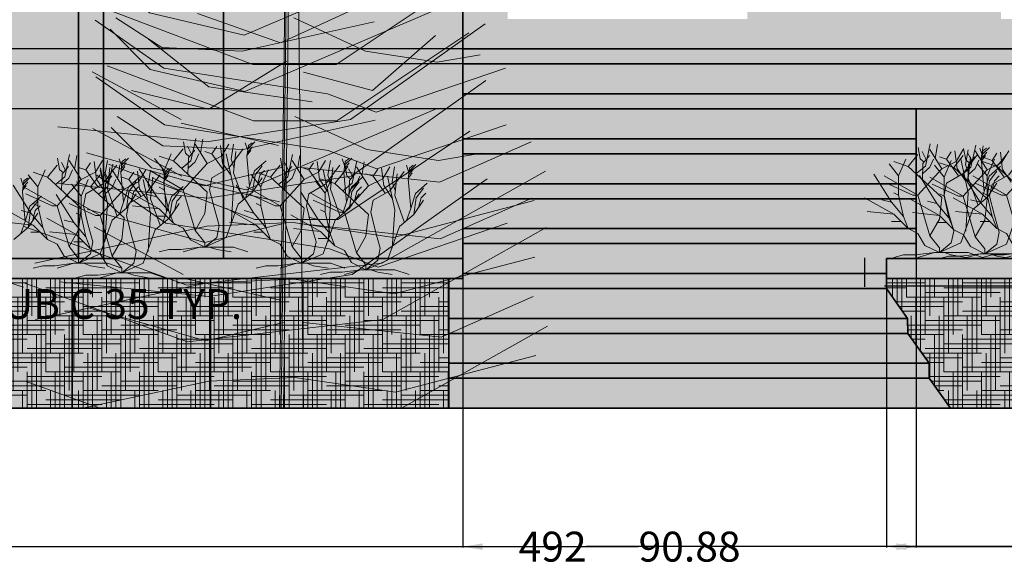
# Model space of a CAD drawing. Units: inches. Extents: x 221 to 874, y 171 to 738.
# Tile 5 of 11: x 452 to 650, y 171 to 281. Entities that reach past the tile are written whole.
import ezdxf

# ---------------------------------------------------------------- set-up
doc = ezdxf.new("R2010")
doc.units = ezdxf.units.IN
doc.header["$MEASUREMENT"] = 0
for name, color, linetype, lineweight in [('A-ANNO-DIMS', 2, 'Continuous', 18), ('A-ELEV', 7, 'Continuous', 35), ('A-ELEV-PATT', 8, 'Continuous', 13), ('L-PLNT', 3, 'Continuous', 13)]:
    doc.layers.add(name, color=color, linetype=linetype, lineweight=lineweight)
doc.styles.get("Standard").update_dxf_attribs({"font": 'arial.ttf'})
doc.dimstyles.get("Standard").update_dxf_attribs({"dimtxt": 6, "dimasz": 4, "dimexe": 0.18, "dimexo": 0.0625, "dimgap": 0.09, "dimtad": 0, "dimtih": 1, "dimtoh": 1, "dimdec": 0, "dimzin": 0, "dimdsep": 46, "dimlunit": 3, "dimtxsty": 'Standard', "dimcen": 0.09, "dimadec": 0, "dimazin": 0, "dimtfac": 1, "dimtdec": 0, "dimtofl": 0, "dimtmove": 0, "dimatfit": 3, "dimfxl": 1, "dimtolj": 1, "dimtzin": 0, "dimarcsym": 0})

# ---------------------------------------------------------------- blocks, each defined once
blk = doc.blocks.new('SHRUB-A')
for p, q in [((8.78, 18.24), (10.7, 20.64)), ((15.5, 17.76), (13.1, 21.6)), ((18.38, 19.2), (19.82, 21.6)), ((19.82, 16.8), (22.7, 20.64)), ((6.86, 16.32), (4.94, 18.72)), ((8.78, 18.24), (5.9, 19.2)), ((6.86, 16.32), (8.3, 19.68)), ((15.5, 12), (8.78, 18.24)), ((10.7, 12.48), (15.5, 17.76)), ((15.5, 17.76), (18.38, 19.2)), ((5.42, 11.04), (1.91, 16.66)), ((10.7, 12.48), (3.98, 16.32)), ((6.86, 12.48), (6.86, 16.32)), ((16.46, 14.88), (19.82, 16.8)), ((25.1, 15.36), (26.54, 17.28)), ((9.74, 12.48), (4.46, 14.88)), ((15.98, 12.48), (16.46, 14.88)), ((24.62, 12), (25.1, 15.36)), ((24.62, 12), (26.54, 14.88)), ((5.9, 8.64), (0, 11.96)), ((6.86, 12.48), (5.9, 12.96)), ((7.82, 8.16), (6.86, 12.48)), ((10.7, 12.48), (9.74, 12.48)), ((13.1, 4.32), (10.7, 12.48)), ((15.02, 7.68), (15.5, 12)), ((16.94, 8.64), (15.98, 12.48)), ((21.74, 9.6), (24.62, 12)), ((5.42, 11.04), (3.5, 11.52)), ((7.82, 8.16), (5.42, 11.04)), ((5.9, 8.64), (0.53, 9.22)), ((8.78, 5.76), (5.9, 8.64)), ((8.78, 5.76), (7.82, 8.16)), ((17.9, 5.28), (16.94, 8.64)), ((19.34, 2.88), (21.74, 9.6)), ((13.1, 4.32), (15.02, 7.68)), ((10.7, 4.8), (8.78, 5.76)), ((12.14, 2.4), (10.7, 4.8)), ((15.02, 1.92), (13.1, 4.32)), ((17.42, 2.88), (17.9, 5.28)), ((15.02, 0.96), (12.14, 2.4)), ((15.02, 0.96), (19.34, 2.88)), ((15.02, 0.96), (17.42, 2.88)), ((15.02, 0.96), (15.02, 1.92)), ((15.02, 0.96), (20.78, 0.96)), ((20.78, 0.96), (23.66, 0))]:
    blk.add_line(p, q)
blk = doc.blocks.new('GRASS-TUFT')
for p, q in [((0.28, 8.35), (0.58, 10.54)), ((0.58, 10.54), (1.31, 11.09)), ((0.83, 2.4), (0.28, 8.35)), ((1.8, 5.45), (4.12, 7.49)), ((0.83, 2.4), (1.8, 5.45)), ((0, 0), (0.83, 2.4))]:
    blk.add_line(p, q)
blk = doc.blocks.new('SHRUB-B')
for p, q in [((8.78, 18.24), (10.7, 20.64)), ((15.5, 17.76), (13.1, 21.6)), ((18.38, 19.2), (19.82, 21.6)), ((19.82, 16.8), (22.7, 20.64)), ((6.86, 16.32), (4.94, 18.72)), ((8.78, 18.24), (5.9, 19.2)), ((6.86, 16.32), (8.3, 19.68)), ((15.5, 12), (8.78, 18.24)), ((10.7, 12.48), (15.5, 17.76)), ((15.5, 17.76), (18.38, 19.2)), ((5.42, 11.04), (1.91, 16.66)), ((10.7, 12.48), (3.98, 16.32)), ((6.86, 12.48), (6.86, 16.32)), ((16.46, 14.88), (19.82, 16.8)), ((25.1, 15.36), (26.54, 17.28)), ((9.74, 12.48), (4.46, 14.88)), ((15.98, 12.48), (16.46, 14.88)), ((24.62, 12), (25.1, 15.36)), ((24.62, 12), (26.54, 14.88)), ((5.9, 8.64), (0, 11.96)), ((6.86, 12.48), (5.9, 12.96)), ((7.82, 8.16), (6.86, 12.48)), ((10.7, 12.48), (9.74, 12.48)), ((13.1, 4.32), (10.7, 12.48)), ((15.02, 7.68), (15.5, 12)), ((16.94, 8.64), (15.98, 12.48)), ((21.74, 9.6), (24.62, 12)), ((5.42, 11.04), (3.5, 11.52)), ((7.82, 8.16), (5.42, 11.04)), ((5.9, 8.64), (0.53, 9.22)), ((8.78, 5.76), (5.9, 8.64)), ((8.78, 5.76), (7.82, 8.16)), ((17.9, 5.28), (16.94, 8.64)), ((19.34, 2.88), (21.74, 9.6)), ((13.1, 4.32), (15.02, 7.68)), ((10.7, 4.8), (8.78, 5.76)), ((12.14, 2.4), (10.7, 4.8)), ((15.02, 1.92), (13.1, 4.32)), ((17.42, 2.88), (17.9, 5.28)), ((15.02, 0.96), (12.14, 2.4)), ((15.02, 0.96), (19.34, 2.88)), ((15.02, 0.96), (17.42, 2.88)), ((15.02, 0.96), (15.02, 1.92)), ((15.02, 0.96), (20.78, 0.96)), ((20.78, 0.96), (23.66, 0)), ((25.58, 0.48), (23.66, 0)), ((27.98, 0.48), (25.58, 0.48)), ((31.82, 0.96), (27.98, 0.48)), ((31.82, 0.96), (28.46, 0)), ((31.82, 0.96), (33.74, 0.96)), ((33.74, 0.96), (35.18, 0.48)), ((35.18, 0.48), (38.06, 0))]:
    blk.add_line(p, q)
blk = doc.blocks.new('GRASS-SPRIG')
for p, q in [((1.44, 3.36), (2.4, 4.8)), ((1.44, 3.36), (0, 3.84)), ((3.84, 0), (1.44, 3.36))]:
    blk.add_line(p, q)
blk = doc.blocks.new('SHRUB-C')
for p, q in [((8.78, 20.16), (10.7, 22.56)), ((15.5, 19.68), (13.1, 23.52)), ((18.38, 21.12), (19.82, 23.52)), ((19.82, 18.72), (22.7, 22.56)), ((6.86, 18.24), (4.94, 20.64)), ((8.78, 20.16), (5.9, 21.12)), ((6.86, 18.24), (8.3, 21.6)), ((15.5, 13.92), (8.78, 20.16)), ((15.5, 19.68), (18.38, 21.12)), ((17.42, 18.24), (19.34, 20.64)), ((24.14, 17.76), (21.74, 21.6)), ((27.02, 19.2), (28.46, 21.6)), ((28.46, 16.8), (31.34, 20.64)), ((5.42, 12.96), (1.91, 18.58)), ((10.7, 14.4), (3.98, 18.24)), ((6.86, 14.4), (6.86, 18.24)), ((10.7, 14.4), (15.5, 19.68)), ((15.5, 16.32), (13.58, 18.72)), ((17.42, 18.24), (14.54, 19.2)), ((15.5, 16.32), (16.94, 19.68)), ((16.46, 16.8), (19.82, 18.72)), ((24.14, 12), (17.42, 18.24)), ((19.34, 12.48), (24.14, 17.76)), ((24.14, 17.76), (27.02, 19.2)), ((25.1, 17.28), (26.54, 19.2)), ((9.74, 14.4), (4.46, 16.8)), ((14.06, 11.04), (10.55, 16.66)), ((19.34, 12.48), (12.62, 16.32)), ((15.5, 12.48), (15.5, 16.32)), ((15.98, 14.4), (16.46, 16.8)), ((24.62, 13.92), (25.1, 17.28)), ((24.62, 13.92), (26.54, 16.8)), ((25.1, 14.88), (28.46, 16.8)), ((33.74, 15.36), (35.18, 17.28)), ((5.9, 10.56), (0, 13.88)), ((6.86, 14.4), (5.9, 14.88)), ((7.82, 10.08), (6.86, 14.4)), ((10.7, 14.4), (9.74, 14.4)), ((13.1, 6.24), (10.7, 14.4)), ((18.38, 12.48), (13.1, 14.88)), ((15.02, 9.6), (15.5, 13.92)), ((16.94, 10.56), (15.98, 14.4)), ((21.74, 11.52), (24.62, 13.92)), ((24.62, 12.48), (25.1, 14.88)), ((33.26, 12), (33.74, 15.36)), ((33.26, 12), (35.18, 14.88)), ((5.42, 12.96), (3.5, 13.44)), ((7.82, 10.08), (5.42, 12.96)), ((14.54, 8.64), (8.64, 11.96)), ((15.5, 12.48), (14.54, 12.96)), ((16.46, 8.16), (15.5, 12.48)), ((19.34, 12.48), (18.38, 12.48)), ((21.74, 4.32), (19.34, 12.48)), ((23.66, 7.68), (24.14, 12)), ((25.58, 8.64), (24.62, 12.48)), ((30.38, 9.6), (33.26, 12)), ((5.9, 10.56), (0.53, 11.14)), ((8.78, 7.68), (5.9, 10.56)), ((8.78, 7.68), (7.82, 10.08)), ((14.06, 11.04), (12.14, 11.52)), ((16.46, 8.16), (14.06, 11.04)), ((17.9, 7.2), (16.94, 10.56)), ((19.34, 4.8), (21.74, 11.52)), ((14.54, 8.64), (9.17, 9.22)), ((13.1, 6.24), (15.02, 9.6)), ((17.42, 5.76), (14.54, 8.64)), ((17.42, 5.76), (16.46, 8.16)), ((26.54, 5.28), (25.58, 8.64)), ((27.98, 2.88), (30.38, 9.6)), ((10.7, 6.72), (8.78, 7.68)), ((12.14, 4.32), (10.7, 6.72)), ((15.02, 3.84), (13.1, 6.24)), ((17.42, 4.8), (17.9, 7.2)), ((21.74, 4.32), (23.66, 7.68)), ((15.02, 2.88), (12.14, 4.32)), ((15.02, 2.88), (19.34, 4.8)), ((15.02, 2.88), (17.42, 4.8)), ((19.34, 4.8), (17.42, 5.76)), ((20.78, 2.4), (19.34, 4.8)), ((23.66, 1.92), (21.74, 4.32)), ((26.06, 2.88), (26.54, 5.28)), ((15.02, 2.88), (15.02, 3.84)), ((15.02, 2.88), (20.78, 2.88)), ((20.78, 2.88), (23.66, 1.92)), ((23.66, 0.96), (20.78, 2.4)), ((23.66, 0.96), (27.98, 2.88)), ((23.66, 0.96), (26.06, 2.88)), ((23.66, 0.96), (23.66, 1.92)), ((23.66, 0.96), (29.42, 0.96)), ((29.42, 0.96), (32.3, 0))]:
    blk.add_line(p, q)
blk = doc.blocks.new('*D16')
at = {"layer": 'A-ANNO-DIMS', "color": 0, "lineweight": -2, "transparency": 16777216}
for p, q in [((621.56, 232.89), (621.56, 227.07)), ((659.62, 232.89), (659.62, 227.07)), ((625.56, 227.25), (655.62, 227.25)), ((659.62, 227.25), (663.62, 227.25))]:
    blk.add_line(p, q, dxfattribs=at)
at = {"layer": 'A-ANNO-DIMS', "color": 0, "transparency": 16777216}
for points in [[(625.56, 227.91), (625.56, 226.58), (621.56, 227.25)], [(655.62, 227.91), (655.62, 226.58), (659.62, 227.25)]]:
    blk.add_solid(points, dxfattribs=at)
at = {"layer": 'Defpoints', "color": 0, "transparency": 16777216}
for p in [(621.56, 232.96), (659.62, 232.96), (659.62, 227.25)]:
    blk.add_point(p, dxfattribs=at)
at = {"layer": 'A-ANNO-DIMS', "color": 0, "transparency": 16777216, "insert": (698.1, 227.25), "char_height": 6, "attachment_point": 5}
blk.add_mtext('\\A1;SHRUB B 38 TYP.', dxfattribs=at)
blk = doc.blocks.new('*D18')
at = {"layer": 'A-ANNO-DIMS', "color": 0, "lineweight": -2, "transparency": 16777216}
for p, q in [((391.06, 228.81), (391.06, 223.42)), ((426.24, 228.81), (426.24, 223.42)), ((395.06, 223.6), (422.24, 223.6)), ((426.24, 223.6), (430.24, 223.6))]:
    blk.add_line(p, q, dxfattribs=at)
at = {"layer": 'A-ANNO-DIMS', "color": 0, "transparency": 16777216}
for points in [[(395.06, 224.27), (395.06, 222.93), (391.06, 223.6)], [(422.24, 224.27), (422.24, 222.93), (426.24, 223.6)]]:
    blk.add_solid(points, dxfattribs=at)
at = {"layer": 'Defpoints', "color": 0, "transparency": 16777216}
for p in [(391.06, 228.88), (426.24, 228.88), (426.24, 223.6)]:
    blk.add_point(p, dxfattribs=at)
at = {"layer": 'A-ANNO-DIMS', "color": 0, "transparency": 16777216, "insert": (464.94, 223.6), "char_height": 6, "attachment_point": 5}
blk.add_mtext('\\A1;SHRUB C 35 TYP.', dxfattribs=at)
blk = doc.blocks.new('*D20')
at = {"layer": 'A-ANNO-DIMS', "color": 0, "lineweight": -2, "transparency": 16777216}
for p, q in [((313.08, 202.65), (313.08, 174.79)), ((805.08, 202.65), (805.08, 174.79)), ((317.08, 174.97), (552.27, 174.97)), ((801.08, 174.97), (565.89, 174.97))]:
    blk.add_line(p, q, dxfattribs=at)
at = {"layer": 'A-ANNO-DIMS', "color": 0, "transparency": 16777216}
for points in [[(317.08, 175.63), (317.08, 174.3), (313.08, 174.97)], [(801.08, 175.63), (801.08, 174.3), (805.08, 174.97)]]:
    blk.add_solid(points, dxfattribs=at)
at = {"layer": 'Defpoints', "color": 0, "transparency": 16777216}
for p in [(313.08, 202.72), (805.08, 202.72), (805.08, 174.97)]:
    blk.add_point(p, dxfattribs=at)
at = {"layer": 'A-ANNO-DIMS', "color": 0, "transparency": 16777216, "insert": (559.08, 174.97), "char_height": 6, "attachment_point": 5}
blk.add_mtext('\\A1;492', dxfattribs=at)
blk = doc.blocks.new('*D21')
at = {"layer": 'A-ANNO-DIMS', "color": 0, "lineweight": -2, "transparency": 16777216}
for p, q in [((541.14, 706.72), (833.01, 706.72)), ((832.83, 702.72), (832.83, 457.87)), ((832.83, 206.72), (832.83, 451.56)), ((805.14, 202.72), (833.01, 202.72))]:
    blk.add_line(p, q, dxfattribs=at)
at = {"layer": 'A-ANNO-DIMS', "color": 0, "transparency": 16777216}
for points in [[(832.16, 702.72), (833.5, 702.72), (832.83, 706.72)], [(832.16, 206.72), (833.5, 206.72), (832.83, 202.72)]]:
    blk.add_solid(points, dxfattribs=at)
at = {"layer": 'Defpoints', "color": 0, "transparency": 16777216}
for p in [(541.08, 706.72), (832.83, 706.72), (805.08, 202.72)]:
    blk.add_point(p, dxfattribs=at)
at = {"layer": 'A-ANNO-DIMS', "color": 0, "transparency": 16777216, "insert": (832.83, 454.72), "char_height": 6, "attachment_point": 5}
blk.add_mtext('\\A1;504', dxfattribs=at)
blk = doc.blocks.new('*D67')
at = {"layer": 'A-ANNO-DIMS', "color": 0, "lineweight": -2, "transparency": 16777216}
for p, q in [((231.54, 271.72), (231.54, 275.72)), ((231.54, 275.72), (235.54, 275.72)), ((541.02, 271.72), (231.36, 271.72)), ((231.54, 266.72), (231.54, 267.72)), ((541.02, 262.72), (231.36, 262.72))]:
    blk.add_line(p, q, dxfattribs=at)
at = {"layer": 'A-ANNO-DIMS', "color": 0, "transparency": 16777216}
for points in [[(230.88, 267.72), (232.21, 267.72), (231.54, 271.72)], [(230.88, 266.72), (232.21, 266.72), (231.54, 262.72)]]:
    blk.add_solid(points, dxfattribs=at)
at = {"layer": 'Defpoints', "color": 0, "transparency": 16777216}
for p in [(231.54, 271.72), (541.08, 271.72), (541.08, 262.72)]:
    blk.add_point(p, dxfattribs=at)
at = {"layer": 'A-ANNO-DIMS', "color": 0, "transparency": 16777216, "insert": (237.61, 275.72), "char_height": 6, "attachment_point": 5}
blk.add_mtext('\\A1;9', dxfattribs=at)
blk = doc.blocks.new('*D68')
at = {"layer": 'A-ANNO-DIMS', "color": 0, "lineweight": -2, "transparency": 16777216}
for p, q in [((231.54, 278.72), (231.54, 282.72)), ((231.54, 282.72), (235.54, 282.72)), ((541.02, 274.72), (231.36, 274.72)), ((541.02, 271.72), (231.36, 271.72)), ((231.54, 267.72), (231.54, 263.72))]:
    blk.add_line(p, q, dxfattribs=at)
at = {"layer": 'A-ANNO-DIMS', "color": 0, "transparency": 16777216}
for points in [[(230.88, 278.72), (232.21, 278.72), (231.54, 274.72)], [(230.88, 267.72), (232.21, 267.72), (231.54, 271.72)]]:
    blk.add_solid(points, dxfattribs=at)
at = {"layer": 'Defpoints', "color": 0, "transparency": 16777216}
for p in [(231.54, 274.72), (541.08, 274.72), (541.08, 271.72)]:
    blk.add_point(p, dxfattribs=at)
at = {"layer": 'A-ANNO-DIMS', "color": 0, "transparency": 16777216, "insert": (237.6, 282.72), "char_height": 6, "attachment_point": 5}
blk.add_mtext('\\A1;3', dxfattribs=at)
blk = doc.blocks.new('*D69')
at = {"layer": 'A-ANNO-DIMS', "color": 0, "lineweight": -2, "transparency": 16777216}
for p, q in [((541.08, 262.65), (541.08, 174.79)), ((631.96, 262.65), (631.96, 174.79)), ((545.08, 174.97), (576.3, 174.97)), ((627.96, 174.97), (596.74, 174.97))]:
    blk.add_line(p, q, dxfattribs=at)
at = {"layer": 'A-ANNO-DIMS', "color": 0, "transparency": 16777216}
for points in [[(545.08, 175.63), (545.08, 174.3), (541.08, 174.97)], [(627.96, 175.63), (627.96, 174.3), (631.96, 174.97)]]:
    blk.add_solid(points, dxfattribs=at)
at = {"layer": 'Defpoints', "color": 0, "transparency": 16777216}
for p in [(541.08, 262.72), (631.96, 262.72), (631.96, 174.97)]:
    blk.add_point(p, dxfattribs=at)
at = {"layer": 'A-ANNO-DIMS', "color": 0, "transparency": 16777216, "insert": (586.52, 174.97), "char_height": 6, "attachment_point": 5}
blk.add_mtext('\\A1;90.88', dxfattribs=at)
blk = doc.blocks.new('*D70')
at = {"layer": 'A-ANNO-DIMS', "color": 0, "lineweight": -2, "transparency": 16777216}
for p, q in [((625.96, 229.65), (625.96, 174.79)), ((805.08, 202.65), (805.08, 174.79)), ((629.96, 174.97), (703.29, 174.97)), ((801.08, 174.97), (727.75, 174.97))]:
    blk.add_line(p, q, dxfattribs=at)
at = {"layer": 'A-ANNO-DIMS', "color": 0, "transparency": 16777216}
for points in [[(629.96, 175.63), (629.96, 174.3), (625.96, 174.97)], [(801.08, 175.63), (801.08, 174.3), (805.08, 174.97)]]:
    blk.add_solid(points, dxfattribs=at)
at = {"layer": 'Defpoints', "color": 0, "transparency": 16777216}
for p in [(625.96, 229.72), (805.08, 202.72), (805.08, 174.97)]:
    blk.add_point(p, dxfattribs=at)
at = {"layer": 'A-ANNO-DIMS', "color": 0, "transparency": 16777216, "insert": (715.52, 174.97), "char_height": 6, "attachment_point": 5}
blk.add_mtext('\\A1;179.12', dxfattribs=at)

msp = doc.modelspace()

# ---------------------------------------------------------------- hatches: boundary and pattern name
at = {"layer": 'A-ELEV-PATT'}
h = msp.add_hatch(color=256, dxfattribs=at)
h.dxf.hatch_style = 1
h.paths.add_polyline_path([(349.0786, 286.1996), (313.0786, 286.1996), (313.0786, 232.7164), (349.0786, 232.7164)])
h.paths.add_polyline_path([(464.0786, 286.1996), (406.0786, 286.1996), (406.0786, 232.7164), (464.0786, 232.7164)])
h.paths.add_polyline_path([(541.0786, 286.1996), (493.0786, 286.1996), (493.0786, 232.7164), (541.0786, 232.7164)])
h.paths.add_polyline_path([(541.0786, 370.7164), (493.0786, 370.7164), (493.0786, 286.1996), (541.0786, 286.1996)])
h.paths.add_polyline_path([(464.0786, 370.7164), (406.0786, 370.7164), (406.0786, 286.1996), (464.0786, 286.1996)])
h.paths.add_polyline_path([(349.0786, 370.7164), (313.0786, 370.7164), (313.0786, 286.1996), (349.0786, 286.1996)])
h.paths.add_polyline_path([(349.0786, 454.7164), (313.0786, 454.7164), (313.0786, 370.7164), (349.0786, 370.7164)])
h.paths.add_polyline_path([(464.0786, 454.7164), (406.0786, 454.7164), (406.0786, 370.7164), (464.0786, 370.7164)])
h.paths.add_polyline_path([(541.0786, 418.7164), (541.0786, 454.7164), (493.0786, 454.7164), (493.0786, 370.7164), (541.0786, 370.7164)])
h.paths.add_polyline_path([(541.0786, 550.7164), (493.0786, 550.7164), (493.0786, 454.7164), (541.0786, 454.7164)])
h.paths.add_polyline_path([(464.0786, 550.7164), (406.0786, 550.7164), (406.0786, 454.7164), (464.0786, 454.7164)])
h.paths.add_polyline_path([(349.0786, 550.7164), (313.0786, 550.7164), (313.0786, 454.7164), (349.0786, 454.7164)])
h.paths.add_polyline_path([(349.0786, 586.7164), (313.0786, 586.7164), (313.0786, 550.7164), (349.0786, 550.7164)])
h.paths.add_polyline_path([(464.0786, 586.7164), (406.0786, 586.7164), (406.0786, 550.7164), (464.0786, 550.7164)])
h.paths.add_polyline_path([(541.0786, 574.7164), (541.0786, 586.7164), (493.0786, 586.7164), (493.0786, 550.7164), (541.0786, 550.7164)])
h.paths.add_polyline_path([(541.0786, 670.7164), (493.0786, 670.7164), (493.0786, 586.7164), (541.0786, 586.7164)])
h.paths.add_polyline_path([(464.0786, 670.7164), (406.0786, 670.7164), (406.0786, 586.7164), (464.0786, 586.7164)])
h.paths.add_polyline_path([(349.0786, 670.7164), (313.0786, 670.7164), (313.0786, 586.7164), (349.0786, 586.7164)])
h.paths.add_polyline_path([(406.0786, 706.7164), (313.0786, 706.7164), (313.0786, 670.7164), (349.0786, 670.7164), (406.0786, 670.7164)])
h.paths.add_polyline_path([(464.0786, 706.7164), (406.0786, 706.7164), (406.0786, 670.7164), (464.0786, 670.7164)])
h.paths.add_polyline_path([(541.0786, 706.7164), (493.0786, 706.7164), (493.0786, 688.7164), (493.0786, 670.7164), (541.0786, 670.7164)])
h.paths.add_polyline_path([(660.0786, 610.7164), (541.0786, 610.7164), (541.0786, 586.7164), (541.0786, 574.7164), (660.0786, 574.7164)])
h.paths.add_polyline_path([(781.0786, 610.7164), (660.0786, 610.7164), (660.0786, 574.7164), (769.0786, 574.7164), (781.0786, 574.7164)])
h.paths.add_polyline_path([(781.0786, 574.7164), (769.0786, 574.7164), (769.0786, 476.1199), (781.0786, 476.1199)])
h.paths.add_polyline_path([(781.0786, 476.1199), (769.0786, 476.1199), (769.0786, 457.7164), (781.0786, 457.7164)])
h.paths.add_polyline_path([(781.0786, 377.1023), (705.9097, 377.1023), (705.9097, 286.1996), (781.0786, 286.1996)])
h.paths.add_polyline_path([(741.9618, 338.8486), (756.9618, 338.8486), (756.9618, 329.8486), (741.9618, 329.8486)], flags=16)
h.paths.add_polyline_path([(648.9097, 377.1023), (598.0786, 377.1023), (598.0786, 286.1996), (648.9097, 286.1996)])
h.paths.add_polyline_path([(781.0786, 286.1996), (705.9097, 286.1996), (705.9097, 280.7164), (648.9097, 280.7164), (648.9097, 286.1996), (598.0786, 286.1996), (598.0786, 280.7164), (550.0786, 280.7164), (550.0786, 286.1996), (541.0786, 286.1996), (541.0786, 274.7164), (781.0786, 274.7164)])
h.paths.add_polyline_path([(660.0786, 562.7164), (546.3477, 562.7164), (546.3477, 457.7164), (660.0786, 457.7164)])
h = msp.add_hatch(color=256, dxfattribs=at)
h.set_gradient(color1=(255, 236, 199), name='CYLINDER')
h.paths.add_polyline_path([(469.0786, 680.7164), (464.0786, 680.7164), (464.0786, 232.7164), (469.0786, 232.7164)])
h = msp.add_hatch(color=256, dxfattribs=at)
h.set_gradient(color1=(99, 100, 102), color2=(254, 234, 185), name='INVCYLINDER')
h.paths.add_polyline_path([(493.0786, 426.7164), (469.0786, 426.7164), (469.0786, 232.7164), (493.0786, 232.7164)])
h = msp.add_hatch(color=256, dxfattribs=at)
h.set_gradient(color1=(99, 100, 102), color2=(169, 160, 132), name='INVCYLINDER')
h.paths.add_polyline_path([(541.0786, 274.7164), (541.0786, 271.7164), (787.0786, 271.7164), (781.0786, 274.7164)])
h = msp.add_hatch(color=256, dxfattribs=at)
h.paths.add_polyline_path([(787.0786, 271.7164), (541.0786, 271.7164), (541.0786, 265.7164), (799.0786, 265.7164)])
h.paths.add_polyline_path([(631.9596, 262.7164), (541.0786, 262.7164), (541.0786, 256.7164), (631.9596, 256.7164)])
h.paths.add_polyline_path([(631.9596, 253.7164), (541.0786, 253.7164), (541.0786, 247.7164), (631.9596, 247.7164)])
h.paths.add_polyline_path([(631.9596, 244.7164), (541.0786, 244.7164), (541.0786, 238.7164), (631.9596, 238.7164)])
h.paths.add_polyline_path([(631.9596, 235.7164), (541.0786, 235.7164), (541.0786, 229.7164), (625.9596, 229.7164), (625.9596, 232.7164), (631.9596, 232.7164)])
h.paths.add_polyline_path([(630.2472, 217.7164), (538.2859, 217.7164), (538.2859, 211.7164), (634.5124, 211.7164), (634.5123, 211.7326)], flags=17)
h.paths.add_polyline_path([(634.5396, 208.7164), (538.2859, 208.7164), (538.2859, 202.7164), (638.8162, 202.7164)])
h = msp.add_hatch(color=256, dxfattribs=at)
h.set_gradient(color1=(99, 100, 102), color2=(248, 246, 176), name='CYLINDER')
h.paths.add_polyline_path([(805.0786, 262.7164), (799.0786, 265.7164), (541.0786, 265.7164), (541.0786, 262.7164)])
for points in [[(631.9596, 262.7164), (631.9596, 232.7164), (805.0786, 232.7164), (805.0786, 262.7164)], [(313.0786, 232.7164), (313.0786, 228.7164), (541.0786, 228.7164), (541.0786, 232.7164)], [(805.0786, 228.7164), (805.0786, 232.7164), (625.9596, 232.7164), (625.9596, 228.7164)], [(538.2859, 226.7164), (538.2859, 220.7164), (630.2279, 220.7164), (625.9626, 226.7164)]]:
    msp.add_hatch(color=256, dxfattribs=at).paths.add_polyline_path(points)
h = msp.add_hatch(color=256, dxfattribs=at)
h.set_gradient(color1=(99, 100, 102), color2=(248, 246, 176), name='CYLINDER')
h.paths.add_polyline_path([(541.0786, 256.7164), (541.0786, 253.7164), (631.9596, 253.7164), (631.9596, 256.7164)])
h = msp.add_hatch(color=256, dxfattribs=at)
h.set_gradient(color1=(99, 100, 102), color2=(248, 246, 176), name='CYLINDER')
h.paths.add_polyline_path([(541.0786, 247.7164), (541.0786, 244.7164), (631.9596, 244.7164), (631.9596, 247.7164)])
h = msp.add_hatch(color=256, dxfattribs=at)
h.set_gradient(color1=(99, 100, 102), color2=(248, 246, 176), name='CYLINDER')
h.paths.add_polyline_path([(631.9596, 235.7164), (631.9596, 238.7164), (541.0786, 238.7164), (541.0786, 235.7164)])
h = msp.add_hatch(color=256, dxfattribs=at)
h.set_gradient(color1=(99, 100, 102), color2=(248, 246, 176), name='CYLINDER')
h.paths.add_polyline_path([(625.9626, 226.7164), (625.9606, 228.7164), (625.9596, 228.7164), (625.9596, 229.7164), (541.0786, 229.7164), (541.0786, 228.7164), (538.2859, 228.7164), (538.2859, 226.7164)])
h = msp.add_hatch(color=256, dxfattribs=at)
h.set_gradient(color1=(147, 149, 152), color2=(91, 91, 91), name='CURVED')
h.paths.add_polyline_path([(462.8078, 202.7164), (462.8078, 228.7164), (414.8291, 228.7164), (414.8291, 202.7164)])
h = msp.add_hatch(dxfattribs=at)
h.set_pattern_fill('HOUND', color=256, scale=15, style=0)
h.paths.add_polyline_path([(462.8078, 228.7164), (414.8291, 228.7164), (414.8291, 202.7164), (462.8078, 202.7164)])
h = msp.add_hatch(color=256, dxfattribs=at)
h.set_gradient(color1=(99, 100, 102), color2=(91, 91, 91), rotation=180, name='INVCURVED')
h.paths.add_polyline_path([(462.8078, 202.7164), (490.5003, 202.7164), (490.5003, 228.7164), (462.8078, 228.7164)])
h = msp.add_hatch(dxfattribs=at)
h.set_pattern_fill('HOUND', color=256, scale=15, style=0)
h.paths.add_polyline_path([(490.5003, 228.7164), (462.8078, 228.7164), (462.8078, 202.7164), (490.5003, 202.7164)])
h = msp.add_hatch(color=256, dxfattribs=at)
h.set_gradient(color1=(147, 149, 152), color2=(91, 91, 91), name='CURVED')
h.paths.add_polyline_path([(538.2859, 202.7164), (538.2859, 228.7164), (490.5003, 228.7164), (490.5003, 202.7164)])
h = msp.add_hatch(dxfattribs=at)
h.set_pattern_fill('HOUND', color=256, scale=15, style=0)
h.paths.add_polyline_path([(538.2859, 228.7164), (490.5003, 228.7164), (490.5003, 202.7164), (538.2859, 202.7164)])
h = msp.add_hatch(color=256, dxfattribs=at)
h.set_gradient(color1=(147, 149, 152), color2=(99, 100, 102), name='CURVED')
h.paths.add_polyline_path([(656.1863, 228.7164), (625.9606, 228.7164), (625.9626, 226.7164), (630.2279, 220.7164), (630.2471, 217.7164), (634.5238, 211.7164), (634.5124, 211.7164), (634.5315, 208.7276), (638.8162, 202.7164), (656.1863, 202.7164)])
h = msp.add_hatch(dxfattribs=at)
h.set_pattern_fill('HOUND', color=256, scale=15, style=0)
h.paths.add_polyline_path([(656.1863, 228.7164), (625.9606, 228.7164), (625.9626, 226.7164), (630.2279, 220.7164), (630.2471, 217.7164), (634.5238, 211.7164), (634.5124, 211.7164), (634.5315, 208.7276), (638.8162, 202.7164), (656.1863, 202.7164)])
h = msp.add_hatch(color=256, dxfattribs=at)
h.set_gradient(color1=(99, 100, 102), color2=(248, 246, 176), name='CYLINDER')
h.paths.add_polyline_path([(630.2471, 217.7164), (630.2279, 220.7164), (538.2859, 220.7164), (538.2859, 217.7164)])
h.paths.add_polyline_path([(634.5316, 208.7164), (634.5124, 211.7164), (538.2859, 211.7164), (538.2859, 208.7164)])

# ---------------------------------------------------------------- linework, layer by layer
at = {"layer": 'A-ELEV'}
for p, q in [((464.0786, 706.7164), (464.0786, 232.7164)), ((493.0786, 688.7164), (493.0786, 232.7164)), ((469.0786, 684.7164), (469.0786, 232.7164)), ((541.0786, 418.7164), (541.0786, 228.7164)), ((781.0786, 274.7164), (541.0786, 274.7164)), ((787.0786, 271.7164), (541.0786, 271.7164)), ((799.0786, 265.7164), (541.0786, 265.7164)), ((805.0786, 262.7164), (541.0786, 262.7164)), ((631.9596, 262.7164), (631.9596, 232.7164)), ((631.9596, 256.7164), (541.0786, 256.7164)), ((631.9596, 253.7164), (541.0786, 253.7164)), ((631.9596, 247.7164), (541.0786, 247.7164)), ((631.9596, 244.7164), (541.0786, 244.7164)), ((631.9596, 238.7164), (541.0786, 238.7164)), ((631.9596, 235.7164), (541.0786, 235.7164)), ((541.0786, 232.7164), (313.0786, 232.7164)), ((469.0786, 232.7164), (464.0786, 232.7164)), ((805.0786, 232.7164), (625.9596, 232.7164)), ((631.9596, 232.7164), (625.9596, 232.7164)), ((625.9596, 232.7164), (625.9596, 228.7164)), ((625.9596, 229.7164), (541.0786, 229.7164)), ((541.0786, 228.7164), (313.0786, 228.7164)), ((462.8078, 228.7164), (462.8078, 202.7164)), ((490.5003, 228.7164), (490.5003, 202.7164)), ((538.2859, 228.7164), (538.2859, 202.7164)), ((805.0786, 228.7164), (625.9596, 228.7164)), ((625.9606, 228.7164), (625.9626, 226.7164)), ((625.9626, 226.7164), (538.2859, 226.7164)), ((625.9626, 226.7164), (630.2279, 220.7164)), ((630.2279, 220.7164), (538.2859, 220.7164)), ((630.2279, 220.7164), (630.2471, 217.7164)), ((630.2472, 217.7164), (538.2859, 217.7164)), ((630.2471, 217.7164), (634.5238, 211.7164)), ((634.5124, 211.7164), (538.2859, 211.7164)), ((634.5124, 211.7164), (634.5316, 208.7165)), ((634.5396, 208.7164), (538.2859, 208.7164)), ((634.5394, 208.7165), (638.8161, 202.7165)), ((805.0786, 202.7164), (313.0786, 202.7164))]:
    msp.add_line(p, q, dxfattribs=at)
msp.add_lwpolyline([(464.0786, 680.7164), (469.0786, 680.7164), (469.0786, 232.7164), (464.0786, 232.7164)], close=True, dxfattribs=at)
at = {"layer": 'L-PLNT'}
for p, q in [((506.7539, 394.7164), (504.3549, 202.7164)), ((506.7539, 394.7164), (509.1549, 202.7164)), ((506.8956, 383.3859), (504.6382, 202.7164)), ((506.8956, 383.3859), (509.1549, 202.7164)), ((507.1423, 363.6628), (505.1313, 202.7164)), ((507.1423, 363.6628), (509.1549, 202.7164)), ((466.7839, 270.1424), (484.6129, 260.5574)), ((466.9256, 258.8119), (484.7546, 249.2269)), ((484.6129, 259.8204), (504.1669, 255.3964)), ((486.5616, 252.3239), (487.5376, 256.7839)), ((488.5146, 253.8099), (489.0026, 256.6269)), ((483.1146, 252.2749), (485.0346, 254.6749)), ((485.5236, 253.8099), (485.0966, 256.0789)), ((486.7146, 253.6539), (485.8906, 255.2189)), ((489.8346, 251.7949), (487.4346, 255.6349)), ((492.9086, 251.7759), (492.4816, 255.3749)), ((492.7146, 253.2349), (494.1546, 255.6349)), ((494.1546, 250.8349), (497.0346, 254.6749)), ((494.6176, 252.6369), (495.1066, 255.6099)), ((497.4866, 255.9229), (497.9136, 254.5929)), ((497.9746, 254.0449), (498.8906, 255.1399)), ((498.0356, 254.7489), (499.3786, 256.0789)), ((536.3729, 248.0234), (554.7769, 256.1334)), ((632.7525, 252.7314), (632.3255, 255.0004)), ((633.7905, 251.2454), (634.7665, 255.7054)), ((635.7435, 252.7314), (636.2315, 255.5484)), ((641.8725, 252.4914), (641.4455, 254.7604)), ((642.9105, 251.0054), (643.8865, 255.4654)), ((644.7155, 254.8444), (645.1425, 253.5144)), ((644.8635, 252.4914), (645.3515, 255.3084)), ((645.2645, 253.6704), (646.6075, 255.0004)), ((460.2476, 250.5714), (459.8206, 252.8404)), ((461.2856, 249.0854), (462.2616, 253.5454)), ((463.2386, 250.5714), (463.7266, 253.3884)), ((465.6339, 253.9214), (489.2129, 247.2854)), ((472.2106, 252.6844), (472.6376, 251.3544)), ((472.7596, 251.5104), (474.1026, 252.8404)), ((481.1946, 250.3549), (479.2746, 252.7549)), ((483.1146, 252.2749), (480.2346, 253.2349)), ((481.1946, 250.3549), (482.6346, 253.7149)), ((486.3176, 253.1059), (485.5236, 253.8099)), ((485.9516, 249.6629), (486.0736, 252.8709)), ((486.0736, 252.8709), (487.3546, 254.4359)), ((487.4156, 252.0889), (488.1486, 253.7319)), ((489.8346, 251.7949), (492.7146, 253.2349)), ((495.1146, 246.9949), (493.6746, 253.7149)), ((495.2286, 250.8369), (494.6176, 252.6369)), ((495.1146, 249.8749), (495.5946, 254.1949)), ((497.8526, 253.4189), (498.5846, 254.4359)), ((504.9488, 250.5714), (504.5218, 252.8404)), ((505.9868, 249.0854), (506.9628, 253.5454)), ((507.9398, 250.5714), (508.4278, 253.3884)), ((516.9118, 252.6844), (517.3388, 251.3544)), ((517.4608, 251.5104), (518.8038, 252.8404)), ((633.5465, 252.0274), (632.7525, 252.7314)), ((633.9435, 252.5754), (633.1195, 254.1404)), ((633.3025, 251.7924), (634.5835, 253.3574)), ((634.6445, 251.0104), (635.3775, 252.6534)), ((640.1375, 250.6974), (639.7105, 254.2964)), ((642.3435, 245.9164), (640.9035, 252.6364)), ((641.8465, 251.5584), (642.3355, 254.5314)), ((643.0635, 252.3354), (642.2395, 253.9004)), ((642.3435, 248.7964), (642.8235, 253.1164)), ((642.4225, 251.5524), (643.7035, 253.1174)), ((645.0815, 252.3404), (645.8135, 253.3574)), ((645.2035, 252.9664), (646.1195, 254.0614)), ((649.2575, 250.4574), (648.8305, 254.0564)), ((461.4386, 250.4154), (460.6146, 251.9804)), ((460.7976, 249.6324), (462.0786, 251.1974)), ((467.6326, 248.5374), (467.2056, 252.1364)), ((468.8876, 248.6514), (468.4606, 250.9204)), ((469.3416, 249.3984), (469.8306, 252.3714)), ((469.8386, 246.6364), (470.3186, 250.9564)), ((469.9256, 247.1654), (470.9016, 251.6254)), ((471.8786, 248.6514), (472.3666, 251.4684)), ((472.5766, 250.1804), (473.3086, 251.1974)), ((472.6986, 250.8064), (473.6146, 251.9014)), ((479.7546, 245.0749), (476.2396, 250.6899)), ((480.8506, 250.7644), (481.2776, 249.4344)), ((481.3996, 249.5904), (482.7426, 250.9204)), ((489.8346, 246.0349), (483.1146, 252.2749)), ((484.6696, 250.7589), (486.5616, 252.3239)), ((485.0346, 246.5149), (489.8346, 251.7949)), ((486.0126, 250.8369), (487.4156, 252.0889)), ((489.2129, 247.2854), (504.7419, 250.9724)), ((490.7946, 248.9149), (494.1546, 250.8349)), ((494.6176, 249.3499), (492.9086, 251.8539)), ((499.4346, 249.3949), (500.8746, 251.3149)), ((506.1398, 250.4154), (505.3158, 251.9804)), ((505.4988, 249.6324), (506.7798, 251.1974)), ((508.7669, 250.9724), (536.3729, 248.0234)), ((510.2198, 250.4764), (508.7798, 250.9564)), ((510.2198, 250.4764), (511.1798, 251.9164)), ((512.3338, 248.5374), (511.9068, 252.1364)), ((514.0428, 249.3984), (514.5318, 252.3714)), ((514.5398, 246.6364), (515.0198, 250.9564)), ((517.2778, 250.1804), (518.0098, 251.1974)), ((517.3998, 250.8064), (518.3158, 251.9014)), ((517.8305, 249.2943), (517.4035, 251.5633)), ((519.0215, 249.1383), (518.1975, 250.7033)), ((518.8685, 247.8083), (519.8445, 252.2683)), ((522.1415, 247.2793), (519.7415, 251.1193)), ((520.8215, 249.2943), (521.3095, 252.1113)), ((525.2155, 247.2603), (524.7885, 250.8593)), ((525.0215, 248.7193), (526.4615, 251.1193)), ((526.9245, 248.1213), (527.4135, 251.0943)), ((529.7935, 251.4073), (530.2205, 250.0773)), ((530.2815, 249.5293), (531.1975, 250.6243)), ((530.3425, 250.2333), (531.6855, 251.5633)), ((631.8985, 249.6804), (633.7905, 251.2454)), ((633.1805, 248.5844), (633.3025, 251.7924)), ((633.2415, 249.7584), (634.6445, 251.0104)), ((641.8465, 248.2714), (640.1375, 250.7754)), ((641.0185, 249.4404), (642.9105, 251.0054)), ((642.4575, 249.7584), (641.8465, 251.5584)), ((642.6665, 251.7874), (641.8725, 252.4914)), ((642.3005, 248.3444), (642.4225, 251.5524)), ((642.3615, 249.5184), (643.7645, 250.7704)), ((643.7645, 250.7704), (644.4975, 252.4134)), ((452.4906, 248.8444), (452.9176, 247.5144)), ((453.0396, 247.6704), (454.3826, 249.0004)), ((459.3936, 247.5204), (461.2856, 249.0854)), ((461.0416, 249.8674), (460.2476, 250.5714)), ((460.6756, 246.4244), (460.7976, 249.6324)), ((460.7366, 247.5984), (462.1396, 248.8504)), ((462.1396, 248.8504), (462.8726, 250.4934)), ((469.8386, 243.7564), (468.3986, 250.4764)), ((469.6816, 247.9474), (468.8876, 248.6514)), ((470.0786, 248.4954), (469.2546, 250.0604)), ((469.9526, 247.5984), (469.3416, 249.3984)), ((469.4376, 247.7124), (470.7186, 249.2774)), ((476.2726, 246.6174), (475.8456, 250.2164)), ((477.9816, 247.4784), (478.4706, 250.4514)), ((485.0346, 246.5149), (478.3146, 250.3549)), ((478.4786, 244.7164), (478.9586, 249.0364)), ((484.0746, 246.5149), (478.7946, 248.9149)), ((481.1946, 246.5149), (481.1946, 250.3549)), ((481.2166, 248.2604), (481.9486, 249.2774)), ((481.3386, 248.8864), (482.2546, 249.9814)), ((490.3146, 246.5149), (490.7946, 248.9149)), ((497.0346, 244.5949), (495.1146, 249.8749)), ((498.9546, 246.0349), (499.4346, 249.3949)), ((498.9546, 246.0349), (500.8746, 248.9149)), ((499.9146, 247.4749), (500.3946, 249.3949)), ((500.3946, 249.3949), (501.3546, 250.3549)), ((504.0948, 247.5204), (505.9868, 249.0854)), ((505.7428, 249.8674), (504.9488, 250.5714)), ((505.3768, 246.4244), (505.4988, 249.6324)), ((505.4378, 247.5984), (506.8408, 248.8504)), ((506.8408, 248.8504), (507.5738, 250.4934)), ((512.6198, 247.1164), (510.2198, 250.4764)), ((515.4215, 247.7593), (512.5415, 248.7193)), ((514.5398, 243.7564), (513.0998, 250.4764)), ((513.5015, 245.8393), (514.9415, 249.1993)), ((514.6538, 247.5984), (514.0428, 249.3984)), ((515.4215, 247.7593), (517.3415, 250.1593)), ((518.6245, 248.5903), (517.8305, 249.2943)), ((518.3805, 248.3553), (519.6615, 249.9203)), ((519.7225, 247.5733), (520.4555, 249.2163)), ((522.1415, 247.2793), (525.0215, 248.7193)), ((527.4215, 242.4793), (525.9815, 249.1993)), ((526.4615, 246.3193), (529.3415, 250.1593)), ((527.4215, 245.3593), (527.9015, 249.6793)), ((530.1595, 248.9033), (530.8915, 249.9203)), ((644.2635, 243.5164), (642.3435, 248.7964)), ((647.6235, 248.3164), (648.5835, 249.2764)), ((650.9665, 248.0314), (649.2575, 250.5354)), ((452.8566, 246.3404), (453.5886, 247.3574)), ((452.9786, 246.9664), (453.8946, 248.0614)), ((469.3416, 246.1114), (467.6326, 248.6154)), ((468.0336, 245.6004), (469.9256, 247.1654)), ((469.3156, 244.5044), (469.4376, 247.7124)), ((469.3766, 245.6784), (470.7796, 246.9304)), ((470.7796, 246.9304), (471.5126, 248.5734)), ((475.1186, 246.1564), (476.0786, 247.1164)), ((477.9816, 244.1914), (476.2726, 246.6954)), ((478.4786, 241.8364), (477.0386, 248.5564)), ((478.5926, 245.6784), (477.9816, 247.4784)), ((481.1946, 246.5149), (480.2346, 246.9949)), ((484.7546, 248.4899), (504.3086, 244.0659)), ((494.6346, 239.3149), (495.1146, 246.9949)), ((513.5015, 245.8393), (511.5815, 248.2393)), ((514.0428, 246.1114), (512.3338, 248.6154)), ((522.1415, 241.5193), (515.4215, 247.7593)), ((516.9765, 246.2433), (518.8685, 247.8083)), ((517.3415, 241.9993), (522.1415, 247.2793)), ((518.2585, 245.1473), (518.3805, 248.3553)), ((518.3195, 246.3213), (519.7225, 247.5733)), ((519.8198, 246.1564), (520.7798, 247.1164)), ((526.9245, 244.8343), (525.2155, 247.3383)), ((527.5355, 246.3213), (526.9245, 248.1213)), ((531.7415, 244.8793), (533.1815, 246.7993)), ((647.1435, 246.3964), (647.6235, 248.3164)), ((471.7586, 241.3564), (469.8386, 246.6364)), ((480.2346, 242.6749), (474.3316, 245.9959)), ((474.6386, 244.2364), (475.1186, 246.1564)), ((479.7546, 245.0749), (477.8346, 245.5549)), ((480.3986, 239.4364), (478.4786, 244.7164)), ((482.1546, 242.1949), (479.7546, 245.0749)), ((482.1546, 242.1949), (481.1946, 246.5149)), ((483.7586, 244.2364), (484.7186, 245.1964)), ((485.0346, 246.5149), (484.0746, 246.5149)), ((487.4346, 238.3549), (485.0346, 246.5149)), ((489.3546, 241.7149), (489.8346, 246.0349)), ((491.2746, 242.6749), (490.3146, 246.5149)), ((496.0746, 243.6349), (498.9546, 246.0349)), ((512.0615, 240.5593), (508.5465, 246.1743)), ((517.3415, 241.9993), (510.6215, 245.8393)), ((513.5015, 241.9993), (513.5015, 245.8393)), ((516.4598, 241.3564), (514.5398, 246.6364)), ((519.3398, 244.2364), (519.8198, 246.1564)), ((523.1015, 244.3993), (526.4615, 246.3193)), ((529.3415, 240.0793), (527.4215, 245.3593)), ((531.2615, 241.5193), (531.7415, 244.8793)), ((532.2215, 242.9593), (532.7015, 244.8793)), ((532.7015, 244.8793), (533.6615, 245.8393)), ((536.5146, 236.6929), (554.9186, 244.8029)), ((641.8635, 238.2364), (642.3435, 245.9164)), ((454.4386, 242.3164), (455.8786, 244.2364)), ((455.3986, 242.3164), (456.3586, 243.2764)), ((469.3586, 236.0764), (469.8386, 243.7564)), ((480.2346, 242.6749), (474.8666, 243.2569)), ((483.2786, 242.3164), (483.7586, 244.2364)), ((493.6746, 236.9149), (496.0746, 243.6349)), ((516.3815, 241.9993), (511.1015, 244.3993)), ((514.0598, 236.0764), (514.5398, 243.7564)), ((522.6215, 241.9993), (523.1015, 244.3993)), ((531.2615, 241.5193), (533.1815, 244.3993)), ((453.9586, 238.9564), (454.4386, 242.3164)), ((453.9586, 238.9564), (455.8786, 241.8364)), ((454.9186, 240.3964), (455.3986, 242.3164)), ((465.7756, 242.5909), (489.3546, 235.9549)), ((477.9986, 234.1564), (478.4786, 241.8364)), ((481.6746, 241.2349), (479.7546, 241.2349)), ((483.1146, 239.7949), (480.2346, 242.6749)), ((483.1146, 239.7949), (482.1546, 242.1949)), ((487.4346, 238.3549), (489.3546, 241.7149)), ((492.2346, 239.3149), (491.2746, 242.6749)), ((512.5415, 238.1593), (506.6385, 241.4803)), ((512.0615, 240.5593), (510.1415, 241.0393)), ((513.5015, 241.9993), (512.5415, 242.4793)), ((514.4615, 237.6793), (513.5015, 241.9993)), ((517.3415, 241.9993), (516.3815, 241.9993)), ((519.7415, 233.8393), (517.3415, 241.9993)), ((521.6615, 237.1993), (522.1415, 241.5193)), ((523.5815, 238.1593), (522.6215, 241.9993)), ((526.9415, 234.7993), (527.4215, 242.4793)), ((528.3815, 239.1193), (531.2615, 241.5193)), ((451.0786, 236.5564), (453.9586, 238.9564)), ((467.1723, 239.0888), (485.0013, 229.5038)), ((485.0346, 238.8349), (483.1146, 239.7949)), ((486.4746, 236.4349), (485.0346, 238.8349)), ((489.3546, 235.9549), (504.8836, 239.6419)), ((491.7546, 236.9149), (492.2346, 239.3149)), ((508.9086, 239.6419), (536.5146, 236.6929)), ((514.4615, 237.6793), (512.0615, 240.5593)), ((525.9815, 232.3993), (528.3815, 239.1193)), ((628.9035, 240.1564), (626.9835, 240.1564)), ((638.0235, 239.9164), (636.1035, 239.9164)), ((646.6635, 240.1564), (644.7435, 240.1564)), ((456.3986, 237.9964), (454.4786, 237.9964)), ((489.3546, 235.9549), (487.4346, 238.3549)), ((489.3546, 234.9949), (493.6746, 236.9149)), ((489.3546, 234.9949), (491.7546, 236.9149)), ((501.0998, 237.9964), (499.1798, 237.9964)), ((512.5415, 238.1593), (507.1735, 238.7413)), ((515.4215, 235.2793), (512.5415, 238.1593)), ((515.4215, 235.2793), (514.4615, 237.6793)), ((519.7415, 233.8393), (521.6615, 237.1993)), ((524.5415, 234.7993), (523.5815, 238.1593)), ((465.0386, 236.0764), (463.1186, 236.0764)), ((488.3946, 234.9949), (484.5546, 234.5149)), ((488.3946, 234.9949), (485.0346, 234.0349)), ((489.3546, 234.9949), (486.4746, 236.4349)), ((488.3946, 234.9949), (490.3146, 234.9949)), ((489.3546, 234.9949), (489.3546, 235.9549)), ((489.3546, 234.9949), (495.1146, 234.9949)), ((490.3146, 234.9949), (491.7546, 234.5149)), ((495.1146, 234.9949), (497.9946, 234.0349)), ((513.9815, 236.7193), (512.0615, 236.7193)), ((517.3415, 234.3193), (515.4215, 235.2793)), ((482.1546, 234.5149), (480.2346, 234.0349)), ((484.5546, 234.5149), (482.1546, 234.5149)), ((491.7546, 234.5149), (494.6346, 234.0349)), ((518.7815, 231.9193), (517.3415, 234.3193)), ((521.6615, 231.4393), (519.7415, 233.8393)), ((524.0615, 232.3993), (524.5415, 234.7993)), ((629.3835, 233.4364), (627.4635, 232.9564)), ((631.7835, 233.4364), (629.3835, 233.4364)), ((635.6235, 233.9164), (631.7835, 233.4364)), ((635.6235, 233.9164), (632.2635, 232.9564)), ((635.6235, 233.9164), (637.5435, 233.9164)), ((638.5035, 233.1964), (636.5835, 232.7164)), ((637.5435, 233.9164), (638.9835, 233.4364)), ((640.9035, 233.1964), (638.5035, 233.1964)), ((638.9835, 233.4364), (641.8635, 232.9564)), ((644.7435, 233.6764), (640.9035, 233.1964)), ((644.7435, 233.6764), (641.3835, 232.7164)), ((644.7435, 233.6764), (646.6635, 233.6764)), ((646.6635, 233.6764), (648.1035, 233.1964)), ((648.1035, 233.1964), (650.9835, 232.7164)), ((456.8786, 231.2764), (454.9586, 230.7964)), ((459.2786, 231.2764), (456.8786, 231.2764)), ((463.1186, 231.7564), (459.2786, 231.2764)), ((463.1186, 231.7564), (459.7586, 230.7964)), ((463.1186, 231.7564), (465.0386, 231.7564)), ((465.0386, 231.7564), (466.4786, 231.2764)), ((466.4786, 231.2764), (469.3586, 230.7964)), ((501.5798, 231.2764), (499.6598, 230.7964)), ((503.9798, 231.2764), (501.5798, 231.2764)), ((507.8198, 231.7564), (503.9798, 231.2764)), ((507.8198, 231.7564), (504.4598, 230.7964)), ((507.8198, 231.7564), (509.7398, 231.7564)), ((509.7398, 231.7564), (511.1798, 231.2764)), ((511.1798, 231.2764), (514.0598, 230.7964)), ((521.6615, 230.4793), (518.7815, 231.9193)), ((521.6615, 230.4793), (525.9815, 232.3993)), ((521.6615, 230.4793), (524.0615, 232.3993)), ((521.6615, 230.4793), (521.6615, 231.4393)), ((465.5186, 229.3564), (463.5986, 228.8764)), ((467.9186, 229.3564), (465.5186, 229.3564)), ((471.7586, 229.8364), (467.9186, 229.3564)), ((471.7586, 229.8364), (468.3986, 228.8764)), ((471.7586, 229.8364), (473.6786, 229.8364)), ((473.6786, 229.8364), (475.1186, 229.3564)), ((475.1186, 229.3564), (477.9986, 228.8764)), ((514.4615, 229.9993), (512.5415, 229.5193)), ((516.8615, 229.9993), (514.4615, 229.9993)), ((520.7015, 230.4793), (516.8615, 229.9993)), ((520.7015, 230.4793), (517.3415, 229.5193)), ((520.7015, 230.4793), (522.6215, 230.4793)), ((521.6615, 230.4793), (527.4215, 230.4793)), ((522.6215, 230.4793), (524.0615, 229.9993)), ((524.0615, 229.9993), (526.9415, 229.5193)), ((527.4215, 230.4793), (530.3015, 229.5193)), ((450.1186, 227.9164), (452.9986, 226.9564)), ((485.0013, 228.7668), (504.5553, 224.3428)), ((536.7613, 216.9698), (555.1653, 225.0798)), ((466.0223, 222.8678), (489.6013, 216.2318)), ((489.6013, 216.2318), (505.1303, 219.9188)), ((509.1553, 219.9188), (536.7613, 216.9698))]:
    msp.add_line(p, q, dxfattribs=at)
for points in [[(470.2349, 290.0494), (478.2859, 281.9394), (497.2649, 277.5154), (535.2229, 293.7364)], [(469.6589, 282.6764), (498.9899, 271.6174), (515.6689, 271.6174), (542.1239, 289.3124)], [(487.8763, 281.8528), (504.5553, 275.9538), (525.2593, 285.5388)], [(470.3766, 278.7189), (478.4276, 270.6089), (497.4066, 266.1849), (535.3646, 282.4059)], [(467.3589, 280.4644), (481.1619, 270.8794), (513.9429, 265.7184), (523.7199, 262.0324), (549.6009, 270.8794)], [(471.5266, 280.9309), (480.7286, 275.0329), (496.8316, 274.2949), (523.2866, 280.1939)], [(507.1836, 280.9309), (521.5616, 274.2949), (535.9396, 272.0829), (544.5666, 273.5579)], [(459.8829, 259.0824), (489.7889, 256.1334), (518.5439, 260.5574), (545.5749, 279.7274)], [(469.8006, 271.3459), (499.1316, 260.2869), (515.8106, 260.2869), (542.2656, 277.9819)], [(478.0993, 276.6908), (490.1773, 267.1058), (510.8813, 264.1568)], [(509.1553, 270.0558), (522.9583, 266.3688), (535.6113, 277.4288)], [(474.6483, 266.3688), (490.1773, 262.6828), (505.7053, 272.2678)], [(460.0246, 247.7519), (489.9306, 244.8029), (518.6856, 249.2269), (545.7166, 268.3969)], [(467.5006, 269.1339), (481.3036, 259.5489), (514.0846, 254.3879), (523.8616, 250.7019), (549.7426, 259.5489)], [(470.6233, 258.9958), (478.6743, 250.8858), (497.6533, 246.4618), (535.6113, 262.6828)], [(471.7733, 261.2078), (480.9753, 255.3098), (497.0783, 254.5718), (523.5333, 260.4708)], [(507.4303, 261.2078), (521.8083, 254.5718), (536.1863, 252.3598), (544.8133, 253.8348)], [(470.0473, 251.6228), (499.3783, 240.5638), (516.0573, 240.5638), (542.5123, 258.2588)], [(452.9809, 239.1754), (485.7629, 227.3784), (524.8709, 231.8024), (557.6519, 250.2354)], [(460.2713, 228.0288), (490.1773, 225.0798), (518.9323, 229.5038), (545.9633, 248.6738)], [(467.7473, 249.4108), (481.5503, 239.8258), (514.3313, 234.6648), (524.1083, 230.9788), (549.9893, 239.8258)], [(455.2819, 231.8024), (489.7889, 239.1754), (507.0419, 239.9124), (527.1709, 236.9634), (555.3519, 244.3364)], [(453.1226, 227.8449), (485.9046, 216.0479), (525.0126, 220.4719), (557.7936, 238.9049)], [(455.4236, 220.4719), (489.9306, 227.8449), (507.1836, 228.5819), (527.3126, 225.6329), (555.4936, 233.0059)], [(528.7584, 202.7164), (558.0403, 219.1818)], [(464.879, 202.7164), (490.1773, 208.1218), (507.4303, 208.8588), (527.5593, 205.9098), (555.7403, 213.2828)], [(453.3693, 208.1218), (468.39, 202.7164)]]:
    msp.add_lwpolyline(points, dxfattribs=at)

# ---------------------------------------------------------------- block references
for name, p in [('GRASS-SPRIG', (489.355, 250.3545)), ('GRASS-TUFT', (497.515, 244.8345)), ('GRASS-TUFT', (644.7439, 243.756)), ('GRASS-TUFT', (472.239, 241.596)), ('GRASS-TUFT', (516.9402, 241.596)), ('SHRUB-B', (621.561, 232.956)), ('SHRUB-A', (630.6808, 232.716)), ('GRASS-SPRIG', (636.5839, 249.276)), ('SHRUB-A', (639.3208, 232.956)), ('GRASS-SPRIG', (645.7039, 249.036)), ('SHRUB-C', (449.056, 228.876)), ('GRASS-SPRIG', (464.079, 247.116)), ('GRASS-TUFT', (480.879, 239.676)), ('SHRUB-A', (493.757, 230.796)), ('GRASS-SPRIG', (521.6619, 245.8389)), ('GRASS-TUFT', (529.8219, 240.3189)), ('GRASS-TUFT', (452.519, 237.756)), ('GRASS-SPRIG', (472.719, 245.196))]:
    msp.add_blockref(name, p, dxfattribs=at)

# ---------------------------------------------------------------- dimensions: what is measured, and where the dimension line sits
at = {"layer": 'A-ANNO-DIMS'}
for base, p1, p2, picture, middle in [((832.8286, 706.7164), (805.0786, 202.7164), (541.0786, 706.7164), '*D21', (832.8286, 454.7164)), ((231.5426, 274.7164), (541.0786, 271.7164), (541.0786, 274.7164), '*D68', (237.5972, 282.7164)), ((231.5426, 271.7164), (541.0786, 262.7164), (541.0786, 271.7164), '*D67', (237.6053, 275.7164))]:
    dim = msp.add_linear_dim(base=base, p1=p1, p2=p2, angle=90, dimstyle='Standard', override={"dimdec": 0, "dimlfac": 1, "dimrnd": 0, "dimzin": 0, "dimdsep": 46, "dimlunit": 2}, dxfattribs=at)
    dim.commit()
    dim.dimension.update_dxf_attribs({"geometry": picture, "text_midpoint": middle})
for base, p1, p2, override, picture, middle in [((631.9596, 174.9664), (541.0786, 262.7164), (631.9596, 262.7164), {"dimdec": 2, "dimlfac": 1, "dimrnd": 0, "dimzin": 0, "dimdsep": 46, "dimlunit": 2}, '*D69', (586.5191, 174.9664)), ((805.0786, 174.9664), (625.9596, 229.7164), (805.0786, 202.7164), {"dimdec": 2, "dimlfac": 1, "dimrnd": 0, "dimzin": 0, "dimdsep": 46, "dimlunit": 2}, '*D70', (715.5191, 174.9664)), ((805.0786, 174.9664), (313.0786, 202.7164), (805.0786, 202.7164), {"dimdec": 0, "dimlfac": 1, "dimrnd": 0, "dimzin": 0, "dimdsep": 46, "dimlunit": 2}, '*D20', (559.0786, 174.9664))]:
    dim = msp.add_linear_dim(base=base, p1=p1, p2=p2, dimstyle='Standard', override=override, dxfattribs=at)
    dim.commit()
    dim.dimension.update_dxf_attribs({"geometry": picture, "text_midpoint": middle})
for base, p1, p2, text, picture, middle in [((659.6235, 227.2469), (621.5605, 232.9564), (659.6235, 232.9564), 'SHRUB B <> TYP.', '*D16', (698.0969, 227.2469)), ((426.2386, 223.5989), (391.0556, 228.8764), (426.2386, 228.8764), 'SHRUB C <> TYP.', '*D18', (464.9432, 223.5989))]:
    dim = msp.add_linear_dim(base=base, p1=p1, p2=p2, text=text, dimstyle='Standard', override={"dimdec": 0, "dimrnd": 0, "dimzin": 0, "dimlunit": 2}, dxfattribs=at)
    dim.commit()
    dim.dimension.update_dxf_attribs({"geometry": picture, "text_midpoint": middle})

doc.saveas('drawing.dxf')
